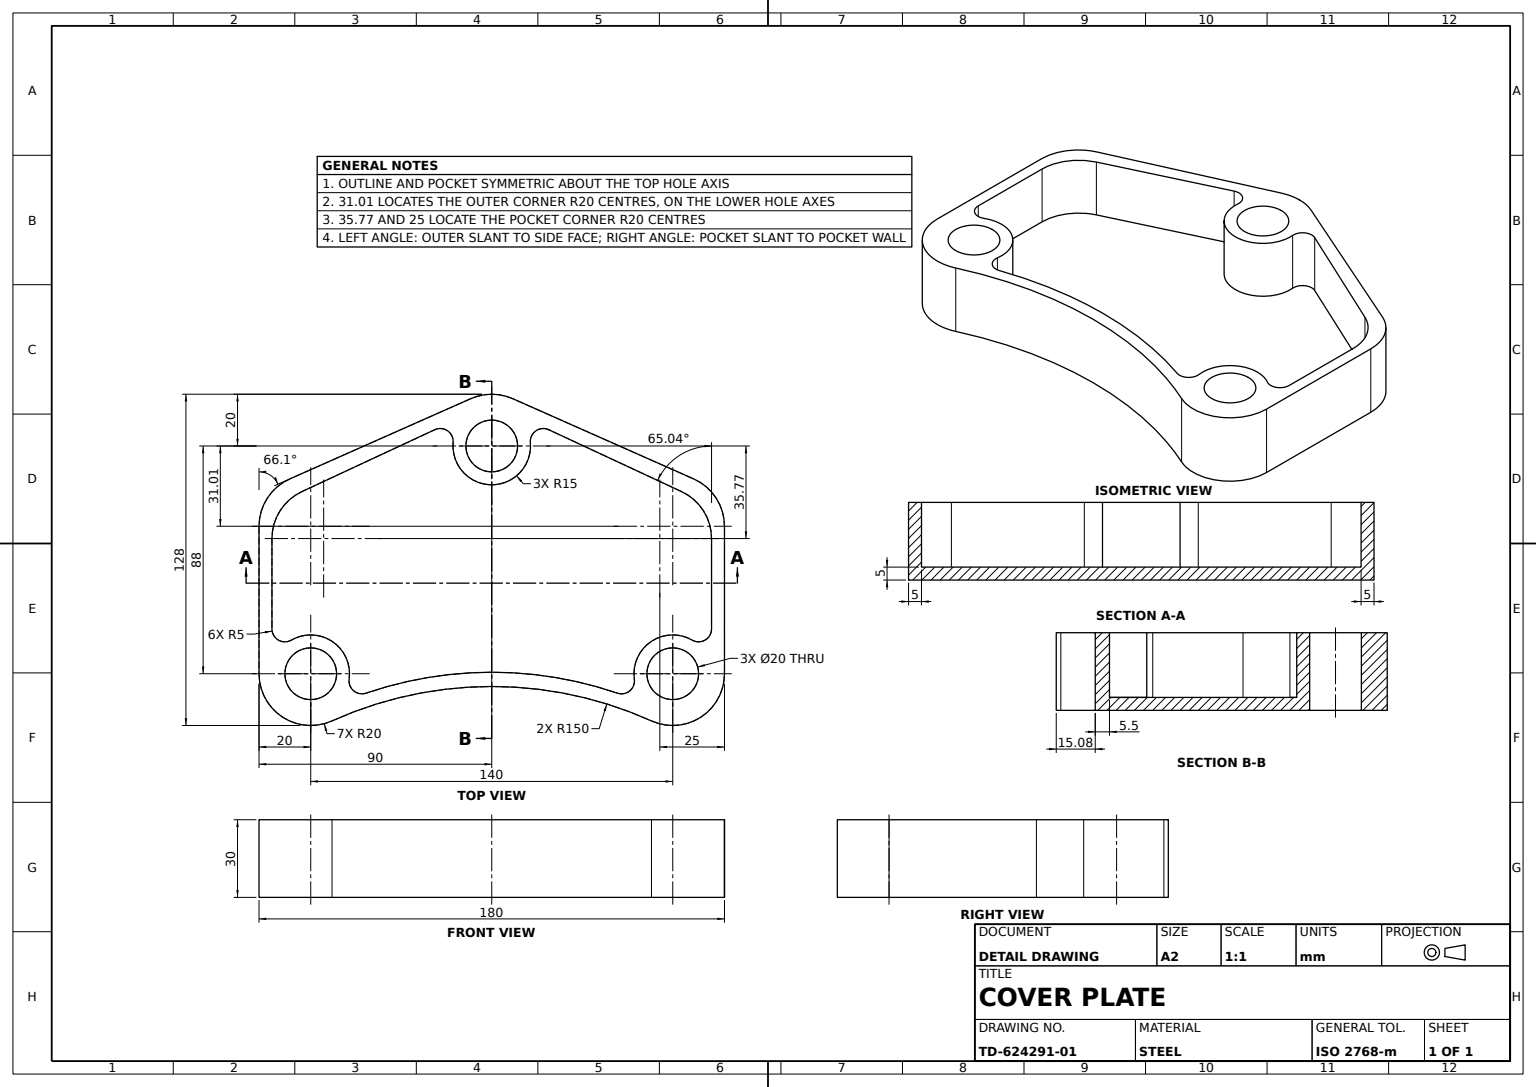
SolidWorks part; units mm, degrees
material "Plain Carbon Steel"
ref_plane "Front Plane" through (0, 0, 0) normal (0, 0, 1) x (1, 0, 0)
ref_plane "Top Plane" through (0, 0, 0) normal (0, 1, 0) x (1, 0, 0)
ref_plane "Right Plane" through (0, 0, 0) normal (1, 0, 0) x (0, 0, -1)
sketch "Plate Outline Sketch" plane through (0, 0, 0) normal (0, 1, 0) x (1, 0, 0)
  line L5 (-85, -35.771) -> (-85, -70.6795)
  line L6 (-90, -31.014) -> (-90, -88)
  line L7 (-73.44, -17.6391) -> (-22.0327, 6.2897)
  line L8 (73.44, -17.6391) -> (22.0327, 6.2897)
  line L9 (8.1016, 18.2856) -> (78.1016, -12.7283)
  line L10 (90, -31.014) -> (90, -88)
  line L12 (-8.1016, 18.2856) -> (-78.1016, -12.7283)
  line L13 (-50.0654, -88) -> (-50, -88) construction
  line L20 (85, -35.771) -> (85, -70.6795)
  circle A0 centre (0, 0) radius 10
  arc A1 (-14.942, 1.3176) -> (14.942, 1.3176) centre (0, 0) ccw
  circle A2 centre (-70, -88) radius 10
  circle A3 centre (70, -88) radius 10
  arc A4 (-55.1443, -90.0754) -> (-77.5, -75.0096) centre (-70, -88) ccw
  arc A5 (-90, -88) -> (-61.7647, -106.2258) centre (-70, -88) ccw
  arc A6 (55.1443, -90.0754) -> (77.5, -75.0096) centre (70, -88) cw
  arc A7 (90, -88) -> (61.7647, -106.2258) centre (70, -88) cw
  arc A9 (90, -31.014) -> (78.1016, -12.7283) centre (70, -31.014) ccw
  arc A10 (-73.44, -17.6391) -> (-85, -35.771) centre (-65, -35.771) ccw
  arc A12 (-77.5, -75.0096) -> (-85, -70.6795) centre (-80, -70.6795) cw
  arc A13 (-22.0327, 6.2897) -> (-14.942, 1.3176) centre (-19.9227, 1.7567) cw
  arc A14 (-90, -31.014) -> (-78.1016, -12.7283) centre (-70, -31.014) cw
  arc A15 (22.0327, 6.2897) -> (14.942, 1.3176) centre (19.9227, 1.7567) ccw
  arc A16 (73.44, -17.6391) -> (85, -35.771) centre (65, -35.771) cw
  arc A17 (8.1016, 18.2856) -> (-8.1016, 18.2856) centre (0, 0) ccw
  arc A18 (-61.7647, -106.2258) -> (61.7647, -106.2258) centre (0, -242.9193) cw
  arc A19 (77.5, -75.0096) -> (85, -70.6795) centre (80, -70.6795) ccw
  arc A20 (-50.001, -88.2015) -> (-50.0654, -88) centre (-44.4191, -86.3085) cw
  arc A21 (-48.5733, -95.4978) -> (48.5733, -95.4978) centre (0, -237.4155) cw
  arc A22 (-50.001, -88.2015) -> (-50, -88) centre (-70, -88) ccw
  arc A23 (-55.1443, -90.0754) -> (-48.5733, -95.4978) centre (-50.1924, -90.7672) ccw
  arc A24 (55.1443, -90.0754) -> (48.5733, -95.4978) centre (50.1924, -90.7672) cw
  point P4 (0, 0)
  point P8 (0, 0)
  point P16 (-70, 0)
  point P19 (-112.2505, -88)
  point P60 (17.052, 5.8505)
  point P71 (82.5, -75.0096)
  dimension "D1" = 20
  dimension "D2" = 30
  dimension "D5" = 20
  dimension "D6" = 30
  dimension "D7" = 40
  dimension "D9" = 5
  dimension "D11" = 20
  dimension "D8" = 20
  dimension "D12" = 150
  dimension "D13" = 70
  dimension "D14" = 150
  dimension "D15" = 90
  dimension "D10" = 5
  dimension "D16" = 5
  dimension "D22" = 5.8941
  dimension "D3" = 140
  dimension "D4" = 90
  dimension "D17" = 70
  dimension "D18" = 88
  dimension "D19" = 31.014
  dimension "D20" = 35.771
  dimension "D21" = 0.0654
  dimension "D23" = 0.2015
  dimension "D24" = 42.2505
  dimension "D25" = 5.8505
extrude "Base Plate" add sketch "Plate Outline Sketch" along normal blind 30 contours A5 A18 A7 L10 A9 L9 A17 L12 A14 L6 A3 A2 A0 A6 A24 A21 A23 A4 A12 L5 A10 L7 A13 A1 A15 L8 A16 L20 A19
sketch "Pocket Sketch" plane through (0, 0, 0) normal (0, -1, 0) x (1, 0, 0)
  line L4 (-90, 88) -> (-90, 31.014)
  line L5 (-78.1016, 12.7283) -> (-8.1016, -18.2856)
  line L6 (8.1016, -18.2856) -> (78.1016, 12.7283)
  line L7 (90, 31.014) -> (90, 88)
  line L8 (-90, 88) -> (-90, 31.014)
  line L9 (-78.1016, 12.7283) -> (-8.1016, -18.2856)
  line L10 (8.1016, -18.2856) -> (78.1016, 12.7283)
  line L11 (90, 31.014) -> (90, 88)
  circle A0 centre (-70, 88) radius 10
  circle A1 centre (0, 0) radius 10
  circle A2 centre (70, 88) radius 10
  arc A6 (-61.7647, 106.2258) -> (-90, 88) centre (-70, 88) ccw
  arc A7 (-90, 31.014) -> (-78.1016, 12.7283) centre (-70, 31.014) ccw
  arc A8 (-8.1016, -18.2856) -> (8.1016, -18.2856) centre (0, 0) ccw
  arc A9 (78.1016, 12.7283) -> (90, 31.014) centre (70, 31.014) ccw
  arc A10 (90, 88) -> (61.7647, 106.2258) centre (70, 88) ccw
  arc A11 (-61.7647, 106.2258) -> (61.7647, 106.2258) centre (0, 242.9193) ccw
  arc A12 (-61.7647, 106.2258) -> (-90, 88) centre (-70, 88) ccw
  arc A13 (-90, 31.014) -> (-78.1016, 12.7283) centre (-70, 31.014) ccw
  arc A14 (-8.1016, -18.2856) -> (8.1016, -18.2856) centre (0, 0) ccw
  arc A15 (78.1016, 12.7283) -> (90, 31.014) centre (70, 31.014) ccw
  arc A16 (90, 88) -> (61.7647, 106.2258) centre (70, 88) ccw
  arc A17 (-61.7647, 106.2258) -> (61.7647, 106.2258) centre (0, 242.9193) ccw
  dimension "D2" = 20
  dimension "D1" = 0
extrude "Pocket" add sketch "Pocket Sketch" against normal blind 5
